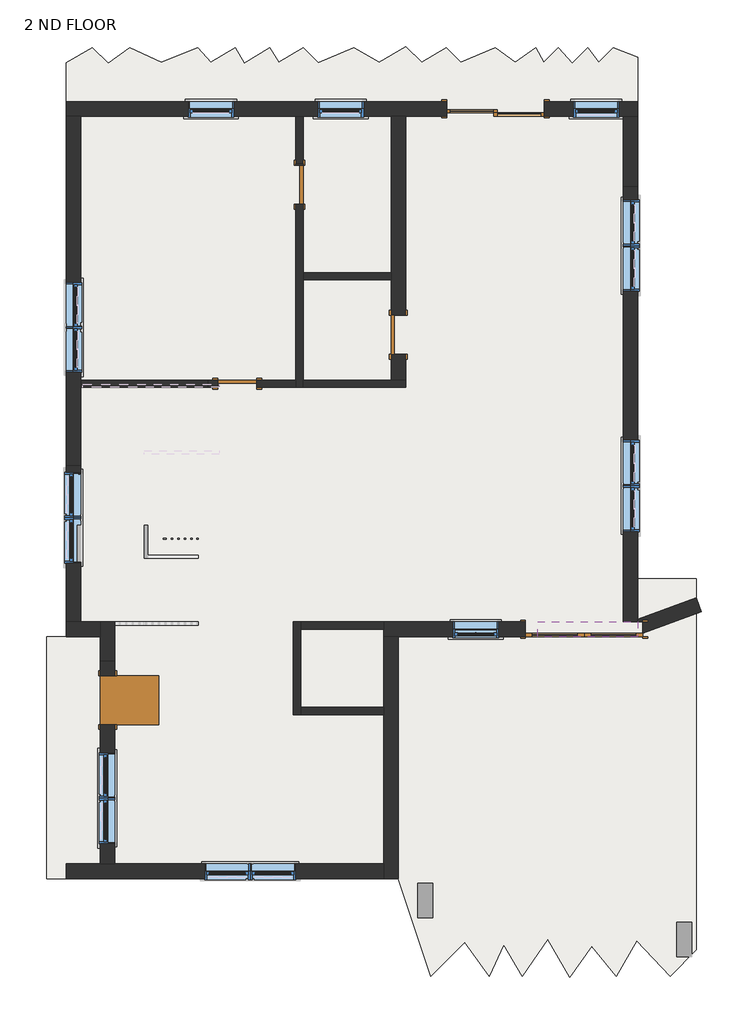
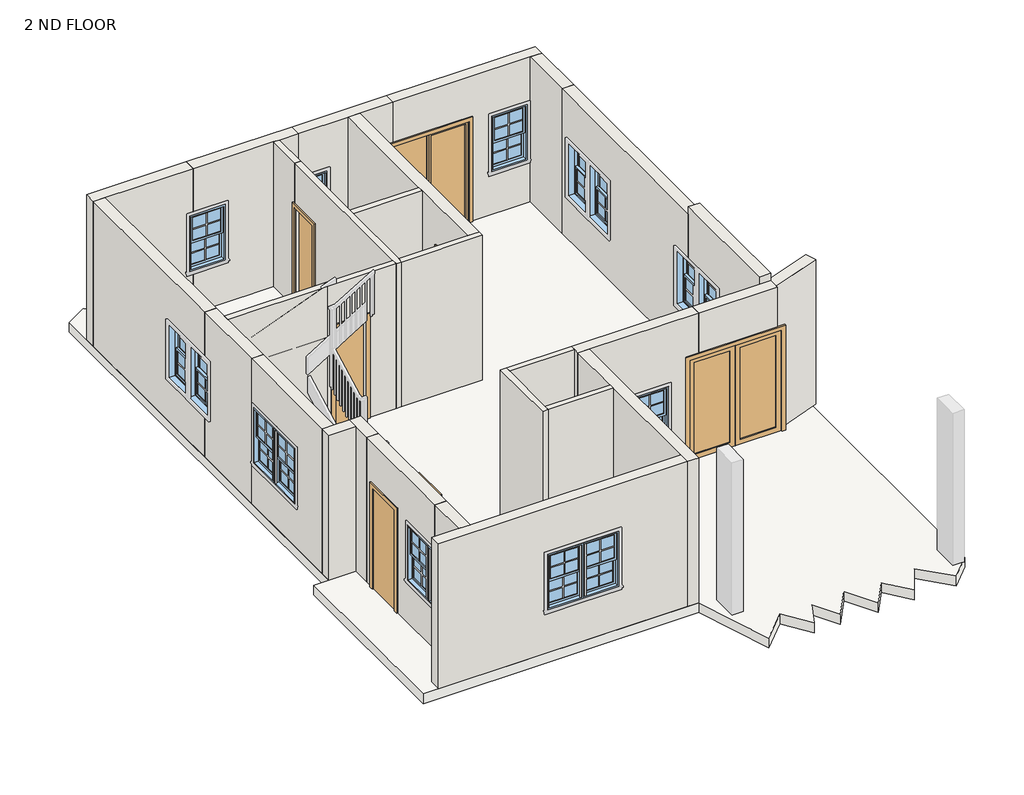
# One storey, part 1 of 3: 29 walls, 16 windows, 6 doors, 1 slab.
"""IFC4 building model written with IfcOpenShell, lengths in millimetres."""

from ifc_helpers import new_model, si_unit, frame, origin, place, context, project, spatial, polyline, outline, extrude, faceted_brep, transform, mapped, element, save
from components import door_5cbd26dd, door_238c678e, single_flush_2_x_7_f433b8c7, door_0bf9f8da, door_0d3b4037, window_fc4bf0c6

model = new_model("IFC4")

# Units and contexts
model_context = context("Model", 3, world=origin())
ifc_project = project(units=[si_unit("LENGTHUNIT", "METRE", prefix="MILLI")], contexts=[model_context])

# Site, building, storey
site = spatial("IfcSite", under=ifc_project)
building = spatial("IfcBuilding", under=site)
storey = spatial("IfcBuildingStorey", under=building, Name="2 ND FLOOR", Elevation=6400.8)

# Doors
placement = place(None, origin())
door_shape = door_5cbd26dd(model_context)
element("IfcDoor", 1, ObjectType="Door-Double-Glass : 72\" x 84\"", at=placement, inside=storey, context=model_context, shape_type="MappedRepresentation", body=[
    mapped(door_shape, transform((-14398.9750992, 4551.4036146, 6400.8), x_axis=(-1.0, 0.0, 0.0), y_axis=(0.0, -1.0, 0.0), z_axis=(0.0, 0.0, 1.0))),
])
door_2_shape = door_238c678e(model_context)
element("IfcDoor", 2, ObjectType="Door-Double-Sliding : 60\" x 84\"", at=placement, inside=storey, context=model_context, shape_type="MappedRepresentation", body=[
    mapped(door_2_shape, transform((-15781.8310804, 12791.3223147, 6400.8), x_axis=(-1.0, 0.0, 0.0), y_axis=(0.0, -1.0, 0.0), z_axis=(0.0, 0.0, 1.0))),
])
single_flush_2_x_7_shape = single_flush_2_x_7_f433b8c7(model_context)
element("IfcDoor", 3, ObjectType="Single-Flush : 2' x 7'", at=placement, inside=storey, context=model_context, shape_type="MappedRepresentation", body=[
    mapped(single_flush_2_x_7_shape, transform((-21828.4750314, 3444.1223646, 6400.8), x_axis=(0.0, 1.0, 0.0), y_axis=(-1.0, 0.0, 0.0), z_axis=(0.0, 0.0, 1.0))),
])
door_3_shape = door_0bf9f8da(model_context)
element("IfcDoor", 4, ObjectType="Single-Flush : 24\" x 84\"", at=placement, inside=storey, context=model_context, shape_type="MappedRepresentation", body=[
    mapped(door_3_shape, transform((-18837.6250314, 11478.1423646, 6400.8), x_axis=(0.0, 1.0, 0.0), y_axis=(-1.0, 0.0, 0.0), z_axis=(0.0, 0.0, 1.0))),
])
element("IfcDoor", 5, ObjectType="Single-Flush : 24\" x 84\"", at=placement, inside=storey, context=model_context, shape_type="MappedRepresentation", body=[
    mapped(door_3_shape, transform((-19809.1750314, 8378.0723646, 6400.8), x_axis=(-1.0, 0.0, 0.0), y_axis=(0.0, -1.0, 0.0), z_axis=(0.0, 0.0, 1.0))),
])
door_4_shape = door_0d3b4037(model_context)
element("IfcDoor", 6, ObjectType="Single-Flush : 24\" x 84\"", at=placement, inside=storey, context=model_context, shape_type="MappedRepresentation", body=[
    mapped(door_4_shape, transform((-17294.5750314, 9140.0723646, 6400.8), x_axis=(0.0, 1.0, 0.0), y_axis=(-1.0, 0.0, 0.0), z_axis=(0.0, 0.0, 1.0))),
])

# Slab
element("IfcSlab", 7, ObjectType="LW Concrete on Metal Deck", at=placement, inside=storey, context=model_context, shape_type="SweptSolid", body=[
    extrude(outline(polyline([(-22065.2814022, 13616.8223646), (-21820.2943548, 13371.8353173), (-21483.0986122, 13616.8223646), (-20992.8643301, 13388.2223646), (-20427.0594754, 13616.8223646), (-20220.0943548, 13388.2223646), (-19839.6400652, 13616.8223646), (-19695.738427, 13377.3298208), (-19297.1559002, 13616.8223646), (-19159.7991627, 13388.2223646), (-18779.344873, 13616.8223646), (-18543.6943548, 13381.1718464), (-17988.5365241, 13616.8223646), (-17592.5897095, 13388.2223646), (-17180.2750314, 13635.9660173), (-16932.5313787, 13388.2223646), (-16552.077089, 13616.8223646), (-16323.477089, 13388.2223646), (-15784.9292382, 13616.8223646), (-15470.2883312, 13388.2223646), (-15155.6474241, 13616.8223646), (-15028.932375, 13388.2223646), (-14800.332375, 13616.8223646), (-14581.2943548, 13373.5559982), (-14338.0279884, 13616.8223646), (-14171.9403665, 13388.2223646), (-13943.3403665, 13616.8223646), (-13560.7750314, 13469.9692914), (-13560.7750314, 5336.4223722), (-12646.3750314, 5336.4223722), (-12646.3750314, -450.2583119), (-13057.2943548, -861.1776354), (-13577.9943548, -311.251504), (-13895.4943548, -861.1776354), (-14276.4943548, -390.1805798), (-14619.3943548, -879.8925313), (-14962.2943548, -285.9723094), (-15365.0574601, -861.1776354), (-15648.0943548, -370.9433534), (-15876.6943548, -861.1776354), (-16257.6943548, -327.7776354), (-16791.0943548, -861.1776354), (-17294.5750314, 662.8223646), (-22780.9751188, 662.8223646), (-22780.9751188, 4434.7223646), (-22476.1752061, 4434.7223646), (-22476.1752061, 13379.5927163), (-22065.2814022, 13616.8223646)])), frame((0.0, 0.0, 6197.6), z_axis=(0.0, 0.0, 1.0), x_axis=(1.0, 0.0, 0.0)), (0.0, 0.0, 1.0), 203.2),
])

# Walls
element("IfcWall", 8, ObjectType="Generic - 4.5\"", at=placement, inside=storey, context=model_context, shape_type="SweptSolid", body=[
    extrude(outline(polyline([(-18894.7750314, 11808.3423646), (-18894.7750314, 12550.0223147), (-18780.4750314, 12550.0223147), (-18780.4750314, 11808.3423646), (-18894.7750314, 11808.3423646)])), frame((0.0, 0.0, 6400.8), z_axis=(0.0, 0.0, 1.0), x_axis=(1.0, 0.0, 0.0)), (0.0, 0.0, 1.0), 3048.0),
])
element("IfcWall", 9, ObjectType="Generic - 4.5\"", at=placement, inside=storey, context=model_context, shape_type="Brep", body=[
    faceted_brep([(-18894.7750314, 11808.3423646, 6400.8), (-18894.7750314, 11782.9423646, 6400.8), (-18894.7750314, 11782.9423646, 8534.4), (-18894.7750314, 11173.3423646, 8534.4), (-18894.7750314, 11173.3423646, 6400.8), (-18894.7750314, 8435.2223646, 6400.8), (-18894.7750314, 8320.9223646, 6400.8), (-18894.7750314, 8320.9223646, 9448.8), (-18894.7750314, 8435.2223646, 9448.8), (-18894.7750314, 11808.3423646, 9448.8), (-18780.4750314, 11782.9423646, 8534.4), (-18780.4750314, 11782.9423646, 6400.8), (-18780.4750314, 11808.3423646, 6400.8), (-18780.4750314, 11808.3423646, 9448.8), (-18780.4750314, 10111.6223646, 9448.8), (-18780.4750314, 9997.3223646, 9448.8), (-18780.4750314, 8435.2223646, 9448.8), (-18780.4750314, 8320.9223646, 9448.8), (-18780.4750314, 8320.9223646, 6400.8), (-18780.4750314, 8435.2223646, 6400.8), (-18780.4750314, 9997.3223646, 6400.8), (-18780.4750314, 10111.6223646, 6400.8), (-18780.4750314, 11173.3423646, 6400.8), (-18780.4750314, 11173.3423646, 8534.4)], [[[0, 1, 2, 3, 4, 5, 6, 7, 8, 9]], [[10, 11, 12, 13, 14, 15, 16, 17, 18, 19, 20, 21, 22, 23]], [[12, 11, 1, 0]], [[22, 21, 20, 19, 18, 6, 5, 4]], [[9, 8, 7, 17, 16, 15, 14, 13]], [[0, 9, 13, 12]], [[7, 6, 18, 17]], [[2, 1, 11, 10]], [[3, 2, 10, 23]], [[4, 3, 23, 22]]]),
])
element("IfcWall", 10, ObjectType="Generic - 4.5\"", at=placement, inside=storey, context=model_context, shape_type="Brep", body=[
    faceted_brep([(-18780.4750314, 8320.9223646, 6400.8), (-17180.2750314, 8320.9223646, 6400.8), (-17180.2750314, 8320.9223646, 9448.8), (-18780.4750314, 8320.9223646, 9448.8), (-18780.4750314, 8435.2223646, 6400.8), (-18780.4750314, 8435.2223646, 9448.8), (-17408.8750314, 8435.2223646, 9448.8), (-17180.2750314, 8435.2223646, 9448.8), (-17180.2750314, 8435.2223646, 6400.8), (-17408.8750314, 8435.2223646, 6400.8)], [[[0, 1, 2, 3]], [[4, 5, 6, 7, 8, 9]], [[1, 0, 4, 9, 8]], [[3, 2, 7, 6, 5]], [[0, 3, 5, 4]], [[2, 1, 8, 7]]]),
])
element("IfcWall", 11, ObjectType="Generic - 4.5\"", at=placement, inside=storey, context=model_context, shape_type="SweptSolid", body=[
    extrude(outline(polyline([(6400.8, -20266.3750314), (6400.8, -20113.9750314), (8534.4, -20113.9750314), (8534.4, -19504.3750314), (6400.8, -19504.3750314), (6400.8, -18894.7750314), (9448.8, -18894.7750314), (9448.8, -20266.3750314), (6400.8, -20266.3750314)])), frame((0.0, 8320.9223646, 0.0), z_axis=(0.0, 1.0, 0.0), x_axis=(0.0, 0.0, 1.0)), (0.0, 0.0, 1.0), 114.3),
])
element("IfcWall", 12, ObjectType="Generic - 4.5\"", at=placement, inside=storey, context=model_context, shape_type="SweptSolid", body=[
    extrude(outline(polyline([(-20266.3750314, 8320.9223646), (-22247.5752061, 8320.9223646), (-22247.5752061, 8435.2223646), (-20266.3750314, 8435.2223646), (-20266.3750314, 8320.9223646)])), frame((0.0, 0.0, 6400.8), z_axis=(0.0, 0.0, 1.0), x_axis=(1.0, 0.0, 0.0)), (0.0, 0.0, 1.0), 3048.0),
])
element("IfcWall", 13, ObjectType="Generic - 4.5\"", at=placement, inside=storey, context=model_context, shape_type="SweptSolid", body=[
    extrude(outline(polyline([(-17408.8750314, 9997.3223646), (-18780.4750314, 9997.3223646), (-18780.4750314, 10111.6223646), (-17408.8750314, 10111.6223646), (-17408.8750314, 9997.3223646)])), frame((0.0, 0.0, 6400.8), z_axis=(0.0, 0.0, 1.0), x_axis=(1.0, 0.0, 0.0)), (0.0, 0.0, 1.0), 3048.0),
])
element("IfcWall", 14, ObjectType="Generic - 4.5\"", at=placement, inside=storey, context=model_context, shape_type="Brep", body=[
    faceted_brep([(-18932.8750314, 4663.3223646, 6400.8), (-18932.8750314, 3215.5223646, 6400.8), (-18932.8750314, 3215.5223646, 9448.8), (-18932.8750314, 4663.3223646, 9448.8), (-18818.5750314, 4663.3223646, 6400.8), (-18818.5750314, 4663.3223646, 9448.8), (-18818.5750314, 4549.0223646, 9448.8), (-18818.5750314, 3329.8223646, 9448.8), (-18818.5750314, 3215.5223646, 9448.8), (-18818.5750314, 3215.5223646, 6400.8), (-18818.5750314, 3329.8223646, 6400.8), (-18818.5750314, 4549.0223646, 6400.8)], [[[0, 1, 2, 3]], [[4, 5, 6, 7, 8, 9, 10, 11]], [[1, 0, 4, 11, 10, 9]], [[3, 2, 8, 7, 6, 5]], [[2, 1, 9, 8]], [[0, 3, 5, 4]]]),
])
element("IfcWall", 15, ObjectType="Generic - 4.5\"", at=placement, inside=storey, context=model_context, shape_type="SweptSolid", body=[
    extrude(outline(polyline([(-17523.1750314, 3215.5223646), (-18818.5750314, 3215.5223646), (-18818.5750314, 3329.8223646), (-17523.1750314, 3329.8223646), (-17523.1750314, 3215.5223646)])), frame((0.0, 0.0, 6400.8), z_axis=(0.0, 0.0, 1.0), x_axis=(1.0, 0.0, 0.0)), (0.0, 0.0, 1.0), 3048.0),
])
element("IfcWall", 16, ObjectType="Generic - 4.5\"", at=placement, inside=storey, context=model_context, shape_type="SweptSolid", body=[
    extrude(outline(polyline([(-17523.1750314, 4549.0223646), (-18818.5750314, 4549.0223646), (-18818.5750314, 4663.3223646), (-17523.1750314, 4663.3223646), (-17523.1750314, 4549.0223646)])), frame((0.0, 0.0, 6400.8), z_axis=(0.0, 0.0, 1.0), x_axis=(1.0, 0.0, 0.0)), (0.0, 0.0, 1.0), 3048.0),
])
element("IfcWall", 17, ObjectType="Generic -9\"Brick 2", at=placement, inside=storey, context=model_context, shape_type="Brep", body=[
    faceted_brep([(-22476.1750314, 12550.0223646, 6400.8), (-22247.5750314, 12550.0223646, 6400.8), (-20494.9750314, 12550.0223646, 6400.8), (-20494.9750314, 12550.0223646, 7315.2), (-20571.1750314, 12550.0223646, 7315.2), (-20571.1750314, 12550.0223646, 8483.6), (-20494.9750314, 12550.0223646, 8483.6), (-20494.9750314, 12550.0223646, 9448.8), (-22247.5750314, 12550.0223646, 9448.8), (-22476.1750314, 12550.0223646, 9448.8), (-20494.9750314, 12778.6223646, 6400.8), (-22476.1750314, 12778.6223646, 6400.8), (-22476.1750314, 12778.6223646, 9448.8), (-20494.9750314, 12778.6223646, 9448.8), (-20494.9750314, 12778.6223646, 8483.6), (-20571.1750314, 12778.6223646, 8483.6), (-20571.1750314, 12778.6223646, 7315.2), (-20494.9750314, 12778.6223646, 7315.2)], [[[0, 1, 2, 3, 4, 5, 6, 7, 8, 9]], [[10, 11, 12, 13, 14, 15, 16, 17]], [[2, 1, 0, 11, 10]], [[2, 10, 17, 3]], [[13, 7, 6, 14]], [[9, 8, 7, 13, 12]], [[0, 9, 12, 11]], [[16, 4, 3, 17]], [[4, 16, 15, 5]], [[5, 15, 14, 6]]]),
])
element("IfcWall", 18, ObjectType="Generic -9\"Brick 2", at=placement, inside=storey, context=model_context, shape_type="Brep", body=[
    faceted_brep([(-20494.9750314, 12550.0223147, 6400.8), (-18894.7750314, 12550.0223147, 6400.8), (-18780.4750314, 12550.0223147, 6400.8), (-18397.0494379, 12550.0223147, 6400.8), (-18397.0494379, 12550.0223147, 7315.2), (-18549.4494379, 12550.0223147, 7315.2), (-18549.4494379, 12550.0223147, 8483.6), (-18397.0494379, 12550.0223147, 8483.6), (-18397.0494379, 12550.0223147, 9448.8), (-18780.4750314, 12550.0223147, 9448.8), (-18894.7750314, 12550.0223147, 9448.8), (-20494.9750314, 12550.0223147, 9448.8), (-20494.9750314, 12550.0223147, 8483.6), (-19859.9750314, 12550.0223147, 8483.6), (-19859.9750314, 12550.0223147, 7315.2), (-20494.9750314, 12550.0223147, 7315.2), (-18397.0494379, 12778.6223147, 6400.8), (-20494.9750314, 12778.6223147, 6400.8), (-20494.9750314, 12778.6223147, 7315.2), (-19859.9750314, 12778.6223147, 7315.2), (-19859.9750314, 12778.6223147, 8483.6), (-20494.9750314, 12778.6223147, 8483.6), (-20494.9750314, 12778.6223147, 9448.8), (-18397.0494379, 12778.6223147, 9448.8), (-18397.0494379, 12778.6223147, 8483.6), (-18549.4494379, 12778.6223147, 8483.6), (-18549.4494379, 12778.6223147, 7315.2), (-18397.0494379, 12778.6223147, 7315.2)], [[[0, 1, 2, 3, 4, 5, 6, 7, 8, 9, 10, 11, 12, 13, 14, 15]], [[16, 17, 18, 19, 20, 21, 22, 23, 24, 25, 26, 27]], [[3, 2, 1, 0, 17, 16]], [[3, 16, 27, 4]], [[23, 8, 7, 24]], [[11, 10, 9, 8, 23, 22]], [[11, 22, 21, 12]], [[17, 0, 15, 18]], [[13, 20, 19, 14]], [[14, 19, 18, 15]], [[20, 13, 12, 21]], [[26, 5, 4, 27]], [[5, 26, 25, 6]], [[6, 25, 24, 7]]]),
])
element("IfcWall", 19, ObjectType="Generic -9\"Brick 2", at=placement, inside=storey, context=model_context, shape_type="Brep", body=[
    faceted_brep([(-16518.4310804, 12550.0223147, 9448.8), (-17180.2750314, 12550.0223147, 9448.8), (-17408.8750314, 12550.0223147, 9448.8), (-18397.0494379, 12550.0223147, 9448.8), (-18397.0494379, 12550.0223147, 8483.6), (-17838.2494379, 12550.0223147, 8483.6), (-17838.2494379, 12550.0223147, 7315.2), (-18397.0494379, 12550.0223147, 7315.2), (-18397.0494379, 12550.0223147, 6400.8), (-17408.8750314, 12550.0223147, 6400.8), (-17180.2750314, 12550.0223147, 6400.8), (-16543.8310804, 12550.0223147, 6400.8), (-16543.8310804, 12550.0223147, 8534.4), (-16518.4310804, 12550.0223147, 8534.4), (-18397.0494379, 12778.6223147, 9448.8), (-16518.4310804, 12778.6223147, 9448.8), (-16518.4310804, 12778.6223147, 8534.4), (-16543.8310804, 12778.6223147, 8534.4), (-16543.8310804, 12778.6223147, 6400.8), (-18397.0494379, 12778.6223147, 6400.8), (-18397.0494379, 12778.6223147, 7315.2), (-17838.2494379, 12778.6223147, 7315.2), (-17838.2494379, 12778.6223147, 8483.6), (-18397.0494379, 12778.6223147, 8483.6)], [[[0, 1, 2, 3, 4, 5, 6, 7, 8, 9, 10, 11, 12, 13]], [[14, 15, 16, 17, 18, 19, 20, 21, 22, 23]], [[8, 19, 18, 11, 10, 9]], [[15, 0, 13, 16]], [[3, 2, 1, 0, 15, 14]], [[3, 14, 23, 4]], [[19, 8, 7, 20]], [[5, 22, 21, 6]], [[6, 21, 20, 7]], [[22, 5, 4, 23]], [[17, 12, 11, 18]], [[12, 17, 16, 13]]]),
])
element("IfcWall", 20, ObjectType="Generic -9\"Brick 2", at=placement, inside=storey, context=model_context, shape_type="Brep", body=[
    faceted_brep([(-13560.7750314, 12550.0223147, 9448.8), (-13789.3750314, 12550.0223147, 9448.8), (-16518.4310804, 12550.0223147, 9448.8), (-16518.4310804, 12550.0223147, 8534.4), (-15019.8310804, 12550.0223147, 8534.4), (-15019.8310804, 12550.0223147, 6400.8), (-13789.3750314, 12550.0223147, 6400.8), (-13560.7750314, 12550.0223147, 6400.8), (-13852.8750314, 12550.0223147, 8483.6), (-13852.8750314, 12550.0223147, 7315.2), (-14564.0750314, 12550.0223147, 7315.2), (-14564.0750314, 12550.0223147, 8483.6), (-16518.4310804, 12778.6223147, 9448.8), (-13560.7750314, 12778.6223147, 9448.8), (-13560.7750314, 12778.6223147, 6400.8), (-15019.8310804, 12778.6223147, 6400.8), (-15019.8310804, 12778.6223147, 8534.4), (-16518.4310804, 12778.6223147, 8534.4), (-13852.8750314, 12778.6223147, 7315.2), (-13852.8750314, 12778.6223147, 8483.6), (-14564.0750314, 12778.6223147, 8483.6), (-14564.0750314, 12778.6223147, 7315.2)], [[[0, 1, 2, 3, 4, 5, 6, 7], [8, 9, 10, 11]], [[12, 13, 14, 15, 16, 17], [18, 19, 20, 21]], [[14, 7, 6, 5, 15]], [[2, 1, 0, 13, 12]], [[2, 12, 17, 3]], [[0, 7, 14, 13]], [[4, 16, 15, 5]], [[16, 4, 3, 17]], [[8, 19, 18, 9]], [[9, 18, 21, 10]], [[10, 21, 20, 11]], [[19, 8, 11, 20]]]),
])
element("IfcWall", 21, ObjectType="Generic -9\"Brick 2", at=placement, inside=storey, context=model_context, shape_type="SweptSolid", body=[
    extrude(outline(polyline([(-13789.3750314, 11447.1098201), (-13789.3750314, 12550.0223147), (-13560.7750314, 12550.0223147), (-13560.7750314, 11447.1098201), (-13789.3750314, 11447.1098201)])), frame((0.0, 0.0, 6400.8), z_axis=(0.0, 0.0, 1.0), x_axis=(1.0, 0.0, 0.0)), (0.0, 0.0, 1.0), 3048.0),
])
element("IfcWall", 22, ObjectType="Generic -9\"Brick 2", at=placement, inside=storey, context=model_context, shape_type="SweptSolid", body=[
    extrude(outline(polyline([(11447.1098201, 6400.8), (7101.7223647, 6400.8), (7101.7223647, 7315.2), (7495.4223646, 7315.2), (7495.4223646, 8483.6), (7101.7223647, 8483.6), (7101.7223647, 9448.8), (11447.1098201, 9448.8), (11447.1098201, 6400.8)]), holes=[polyline([(9821.5098201, 7315.2), (11243.9098201, 7315.2), (11243.9098201, 8483.6), (9821.5098201, 8483.6), (9821.5098201, 7315.2)])]), frame((-13789.3750314, 0.0, 0.0), z_axis=(1.0, 0.0, 0.0), x_axis=(0.0, 1.0, 0.0)), (0.0, 0.0, 1.0), 228.6),
])
element("IfcWall", 23, ObjectType="Generic -9\"Brick 2", at=placement, inside=storey, context=model_context, shape_type="Brep", body=[
    faceted_brep([(-13789.3750314, 7101.7223647, 6400.8), (-13789.3750314, 4663.3223646, 6400.8), (-13789.3750314, 4663.3223646, 9601.2), (-13789.3750314, 7101.7223647, 9601.2), (-13789.3750314, 7101.7223647, 9448.8), (-13789.3750314, 7101.7223647, 8483.6), (-13789.3750314, 6073.0223646, 8483.6), (-13789.3750314, 6073.0223646, 7315.2), (-13789.3750314, 7101.7223647, 7315.2), (-13560.7750314, 4663.3223646, 6400.8), (-13560.7750314, 4704.9241624, 6400.8), (-13560.7750314, 7101.7223647, 6400.8), (-13560.7750314, 7101.7223647, 7315.2), (-13560.7750314, 6073.0223646, 7315.2), (-13560.7750314, 6073.0223646, 8483.6), (-13560.7750314, 7101.7223647, 8483.6), (-13560.7750314, 7101.7223647, 9448.8), (-13560.7750314, 7101.7223647, 9601.2), (-13560.7750314, 4663.3223646, 9601.2), (-13560.7750314, 4663.3223646, 9448.8), (-13560.7750314, 4663.3223646, 8534.4)], [[[0, 1, 2, 3, 4, 5, 6, 7, 8]], [[9, 10, 11, 12, 13, 14, 15, 16, 17, 18, 19, 20]], [[1, 0, 11, 10, 9]], [[3, 2, 18, 17]], [[3, 17, 16, 15, 5, 4]], [[11, 0, 8, 12]], [[2, 1, 9, 20, 19, 18]], [[7, 13, 12, 8]], [[5, 15, 14, 6]], [[13, 7, 6, 14]]]),
])
element("IfcWall", 24, ObjectType="Generic -9\"Brick 2", at=placement, inside=storey, context=model_context, shape_type="Brep", body=[
    faceted_brep([(-13560.7750314, 4434.7223646, 9448.8), (-15122.8751671, 4434.7223646, 9448.8), (-15122.8751671, 4434.7223646, 8534.4), (-13560.7750314, 4434.7223646, 8534.4), (-15122.8751671, 4663.3223646, 9448.8), (-13560.7750314, 4663.3223646, 9448.8), (-13560.7750314, 4663.3223646, 8534.4), (-15122.8751671, 4663.3223646, 8534.4), (-13560.7750314, 4461.6531236, 9448.8), (-13560.7750314, 4461.6531236, 8534.4)], [[[0, 1, 2, 3]], [[4, 5, 6, 7]], [[1, 0, 8, 5, 4]], [[1, 4, 7, 2]], [[5, 8, 0, 3, 9, 6]], [[3, 2, 7, 6, 9]]]),
])
element("IfcWall", 25, ObjectType="Generic -9\"Brick 2", at=placement, inside=storey, context=model_context, shape_type="Brep", body=[
    faceted_brep([(-17523.1750314, 4663.3223722, 9448.8), (-15122.8751671, 4663.3223722, 9448.8), (-15122.8751671, 4663.3223722, 8534.4), (-15313.3750992, 4663.3223722, 8534.4), (-15313.3750992, 4663.3223722, 6400.8), (-17523.1750314, 4663.3223722, 6400.8), (-15732.4750314, 4663.3223722, 6961.9134602), (-15732.4750314, 4663.3223722, 8130.3134602), (-16443.6750314, 4663.3223722, 8130.3134602), (-16443.6750314, 4663.3223722, 6961.9134602), (-15122.8751671, 4434.7223722, 9448.8), (-17294.5750314, 4434.7223722, 9448.8), (-17523.1750314, 4434.7223722, 9448.8), (-17523.1750314, 4434.7223722, 6400.8), (-17294.5750314, 4434.7223722, 6400.8), (-15313.3750992, 4434.7223722, 6400.8), (-15313.3750992, 4434.7223722, 8534.4), (-15122.8751671, 4434.7223722, 8534.4), (-15732.4750314, 4434.7223722, 8130.3134602), (-15732.4750314, 4434.7223722, 6961.9134602), (-16443.6750314, 4434.7223722, 6961.9134602), (-16443.6750314, 4434.7223722, 8130.3134602), (-17523.1750314, 4549.0223646, 6400.8), (-17523.1750314, 4549.0223646, 9448.8)], [[[0, 1, 2, 3, 4, 5], [6, 7, 8, 9]], [[10, 11, 12, 13, 14, 15, 16, 17], [18, 19, 20, 21]], [[13, 22, 5, 4, 15, 14]], [[1, 0, 23, 12, 11, 10]], [[1, 10, 17, 2]], [[0, 5, 22, 13, 12, 23]], [[3, 16, 15, 4]], [[16, 3, 2, 17]], [[18, 7, 6, 19]], [[19, 6, 9, 20]], [[20, 9, 8, 21]], [[7, 18, 21, 8]]]),
])
element("IfcWall", 26, ObjectType="Generic -9\"Brick 2", at=placement, inside=storey, context=model_context, shape_type="Brep", body=[
    faceted_brep([(-17523.1750314, 4434.7223722, 6400.8), (-17523.1750314, 3329.8223646, 6400.8), (-17523.1750314, 3215.5223646, 6400.8), (-17523.1750314, 891.4223646, 6400.8), (-17523.1750314, 662.8223646, 6400.8), (-17523.1750314, 662.8223646, 9448.8), (-17523.1750314, 891.4223646, 9448.8), (-17523.1750314, 3215.5223646, 9448.8), (-17523.1750314, 3329.8223646, 9448.8), (-17523.1750314, 4434.7223722, 9448.8), (-17294.5750314, 4434.7223722, 6400.8), (-17294.5750314, 4434.7223722, 9448.8), (-17294.5750314, 662.8223646, 9448.8), (-17294.5750314, 662.8223646, 6400.8)], [[[0, 1, 2, 3, 4, 5, 6, 7, 8, 9]], [[10, 11, 12, 13]], [[4, 3, 2, 1, 0, 10, 13]], [[9, 8, 7, 6, 5, 12, 11]], [[0, 9, 11, 10]], [[5, 4, 13, 12]]]),
])
element("IfcWall", 27, ObjectType="Generic -9\"Brick 2", at=placement, inside=storey, context=model_context, shape_type="Brep", body=[
    faceted_brep([(-17523.1750314, 891.4223646, 6400.8), (-21714.1750314, 891.4223646, 6400.8), (-21942.7750314, 891.4223646, 6400.8), (-22476.1750314, 891.4223646, 6400.8), (-22476.1750314, 891.4223646, 9448.8), (-21942.7750314, 891.4223646, 9448.8), (-21714.1750314, 891.4223646, 9448.8), (-17523.1750314, 891.4223646, 9448.8), (-18894.6931686, 891.4223646, 8483.6), (-20317.0931686, 891.4223646, 8483.6), (-20317.0931686, 891.4223646, 7315.2), (-18894.6931686, 891.4223646, 7315.2), (-22476.1750314, 662.8223646, 6400.8), (-17523.1750314, 662.8223646, 6400.8), (-17523.1750314, 662.8223646, 9448.8), (-22476.1750314, 662.8223646, 9448.8), (-20317.0931686, 662.8223646, 8483.6), (-18894.6931686, 662.8223646, 8483.6), (-18894.6931686, 662.8223646, 7315.2), (-20317.0931686, 662.8223646, 7315.2)], [[[0, 1, 2, 3, 4, 5, 6, 7], [8, 9, 10, 11]], [[12, 13, 14, 15], [16, 17, 18, 19]], [[3, 2, 1, 0, 13, 12]], [[4, 3, 12, 15]], [[7, 6, 5, 4, 15, 14]], [[0, 7, 14, 13]], [[8, 17, 16, 9]], [[19, 10, 9, 16]], [[17, 8, 11, 18]], [[18, 11, 10, 19]]]),
])
element("IfcWall", 28, ObjectType="Generic -9\"Brick 2", at=placement, inside=storey, context=model_context, shape_type="SweptSolid", body=[
    extrude(outline(polyline([(1710.5723646, 6400.8), (891.4223646, 6400.8), (891.4223646, 9448.8), (1710.5723646, 9448.8), (1710.5723646, 8483.6), (1202.5723646, 8483.6), (1202.5723646, 7315.2), (1710.5723646, 7315.2), (1710.5723646, 6400.8)])), frame((-21942.7750314, 0.0, 0.0), z_axis=(1.0, 0.0, 0.0), x_axis=(0.0, 1.0, 0.0)), (0.0, 0.0, 1.0), 228.6),
])
element("IfcWall", 29, ObjectType="Generic -9\"Brick 2", at=placement, inside=storey, context=model_context, shape_type="SweptSolid", body=[
    extrude(outline(polyline([(1710.5723646, 9448.8), (4053.7223646, 9448.8), (4053.7223646, 6400.8), (3825.1223646, 6400.8), (3825.1223646, 8534.4), (3063.1223646, 8534.4), (3063.1223646, 6400.8), (1710.5723646, 6400.8), (1710.5723646, 7315.2), (2624.9723646, 7315.2), (2624.9723646, 8483.6), (1710.5723646, 8483.6), (1710.5723646, 9448.8)])), frame((-21942.7750314, 0.0, 0.0), z_axis=(1.0, 0.0, 0.0), x_axis=(0.0, 1.0, 0.0)), (0.0, 0.0, 1.0), 228.6),
])
element("IfcWall", 30, ObjectType="Generic -9\"Brick 2", at=placement, inside=storey, context=model_context, shape_type="Brep", body=[
    faceted_brep([(-21714.1750314, 4053.7223646, 6400.8), (-21714.1750314, 4663.3223646, 6400.8), (-21714.1750314, 4663.3223646, 9448.8), (-21714.1750314, 4053.7223646, 9448.8), (-21942.7750314, 4053.7223646, 6400.8), (-21942.7750314, 4053.7223646, 9448.8), (-21942.7750314, 4434.7223646, 9448.8), (-21942.7750314, 4663.3223646, 9448.8), (-21942.7750314, 4663.3223646, 6400.8), (-21942.7750314, 4434.7223646, 6400.8)], [[[0, 1, 2, 3]], [[4, 5, 6, 7, 8, 9]], [[1, 0, 4, 9, 8]], [[3, 2, 7, 6, 5]], [[0, 3, 5, 4]], [[2, 1, 8, 7]]]),
])
element("IfcWall", 31, ObjectType="Generic -9\"Brick 2", at=placement, inside=storey, context=model_context, shape_type="SweptSolid", body=[
    extrude(outline(polyline([(12550.0223646, 6400.8), (8710.539033, 6400.8), (8710.539033, 7315.2), (9955.139033, 7315.2), (9955.139033, 8483.6), (8710.539033, 8483.6), (8710.539033, 9448.8), (12550.0223646, 9448.8), (12550.0223646, 6400.8)])), frame((-22476.1750314, 0.0, 0.0), z_axis=(1.0, 0.0, 0.0), x_axis=(0.0, 1.0, 0.0)), (0.0, 0.0, 1.0), 228.6),
])
element("IfcWall", 32, ObjectType="Generic -9\"Brick 2", at=placement, inside=storey, context=model_context, shape_type="Brep", body=[
    faceted_brep([(-22476.1752061, 8710.539033, 6400.8), (-22476.1752061, 7101.7223643, 6400.8), (-22476.1752061, 7101.7223643, 9448.8), (-22476.1752061, 8710.539033, 9448.8), (-22476.1752061, 8710.539033, 8483.6), (-22476.1752061, 8558.139033, 8483.6), (-22476.1752061, 8558.139033, 7315.2), (-22476.1752061, 8710.539033, 7315.2), (-22247.5752061, 7101.7223643, 6400.8), (-22247.5752061, 8320.9223646, 6400.8), (-22247.5752061, 8435.2223646, 6400.8), (-22247.5752061, 8710.539033, 6400.8), (-22247.5752061, 8710.539033, 7315.2), (-22247.5752061, 8558.139033, 7315.2), (-22247.5752061, 8558.139033, 8483.6), (-22247.5752061, 8710.539033, 8483.6), (-22247.5752061, 8710.539033, 9448.8), (-22247.5752061, 8435.2223646, 9448.8), (-22247.5752061, 8320.9223646, 9448.8), (-22247.5752061, 7101.7223643, 9448.8)], [[[0, 1, 2, 3, 4, 5, 6, 7]], [[8, 9, 10, 11, 12, 13, 14, 15, 16, 17, 18, 19]], [[1, 0, 11, 10, 9, 8]], [[2, 1, 8, 19]], [[3, 2, 19, 18, 17, 16]], [[3, 16, 15, 4]], [[11, 0, 7, 12]], [[6, 13, 12, 7]], [[13, 6, 5, 14]], [[14, 5, 4, 15]]]),
])
element("IfcWall", 33, ObjectType="Generic -9\"Brick 2", at=placement, inside=storey, context=model_context, shape_type="SweptSolid", body=[
    extrude(outline(polyline([(7101.7223643, 6400.8), (4663.3223646, 6400.8), (4663.3223646, 9448.8), (7101.7223643, 9448.8), (7101.7223643, 6400.8)]), holes=[polyline([(5577.7223643, 7315.2), (7000.1223643, 7315.2), (7000.1223643, 8483.6), (5577.7223643, 8483.6), (5577.7223643, 7315.2)])]), frame((-22476.1752061, 0.0, 0.0), z_axis=(1.0, 0.0, 0.0), x_axis=(0.0, 1.0, 0.0)), (0.0, 0.0, 1.0), 228.6),
])
element("IfcWall", 34, ObjectType="Generic -9\"Brick 2", at=placement, inside=storey, context=model_context, shape_type="Brep", body=[
    faceted_brep([(-22476.1752061, 4434.7223646, 6400.8), (-21942.7750314, 4434.7223646, 6400.8), (-21942.7750314, 4434.7223646, 9448.8), (-22476.1752061, 4434.7223646, 9448.8), (-22476.1752061, 4663.3223646, 6400.8), (-22476.1752061, 4663.3223646, 9448.8), (-22247.5752061, 4663.3223646, 9448.8), (-21942.7750314, 4663.3223646, 9448.8), (-21942.7750314, 4663.3223646, 6400.8), (-22247.5752061, 4663.3223646, 6400.8)], [[[0, 1, 2, 3]], [[4, 5, 6, 7, 8, 9]], [[1, 0, 4, 9, 8]], [[3, 2, 7, 6, 5]], [[0, 3, 5, 4]], [[2, 1, 8, 7]]]),
])
element("IfcWall", 35, ObjectType="Generic -9\"Brick 2", at=placement, inside=storey, context=model_context, shape_type="Brep", body=[
    faceted_brep([(-17408.8750314, 12550.0223147, 6400.8), (-17408.8750314, 10111.6223646, 6400.8), (-17408.8750314, 9997.3223646, 6400.8), (-17408.8750314, 9444.8723646, 6400.8), (-17408.8750314, 9444.8723646, 8534.4), (-17408.8750314, 8835.2723646, 8534.4), (-17408.8750314, 8835.2723646, 6400.8), (-17408.8750314, 8435.2223646, 6400.8), (-17408.8750314, 8435.2223646, 9448.8), (-17408.8750314, 9997.3223646, 9448.8), (-17408.8750314, 10111.6223646, 9448.8), (-17408.8750314, 12550.0223147, 9448.8), (-17180.2750314, 9444.8723646, 8534.4), (-17180.2750314, 9444.8723646, 6400.8), (-17180.2750314, 12550.0223147, 6400.8), (-17180.2750314, 12550.0223147, 9448.8), (-17180.2750314, 8435.2223646, 9448.8), (-17180.2750314, 8435.2223646, 6400.8), (-17180.2750314, 8835.2723646, 6400.8), (-17180.2750314, 8835.2723646, 8534.4)], [[[0, 1, 2, 3, 4, 5, 6, 7, 8, 9, 10, 11]], [[12, 13, 14, 15, 16, 17, 18, 19]], [[18, 17, 7, 6]], [[14, 13, 3, 2, 1, 0]], [[11, 10, 9, 8, 16, 15]], [[0, 11, 15, 14]], [[8, 7, 17, 16]], [[4, 3, 13, 12]], [[5, 4, 12, 19]], [[6, 5, 19, 18]]]),
])
element("IfcWall", 36, ObjectType="Generic -9\"Brick 2", at=placement, inside=storey, context=model_context, shape_type="Brep", body=[
    faceted_brep([(-12570.5569462, 4822.063032, 6400.8), (-12570.5569462, 4822.063032, 9448.8), (-13560.7750314, 4461.6531236, 9448.8), (-13560.7750314, 4461.6531236, 8534.4), (-13484.5750992, 4489.3876307, 8534.4), (-13484.5750992, 4489.3876307, 6400.8), (-12648.7427509, 5036.8767651, 6400.8), (-13560.7750314, 4704.9241624, 6400.8), (-13560.7750314, 4704.9241624, 9448.8), (-12648.7427509, 5036.8767651, 9448.8), (-13484.5750992, 4663.3223646, 6400.8), (-13560.7750314, 4663.3223646, 6400.8), (-13560.7750314, 4663.3223646, 9448.8), (-13560.7750314, 4663.3223646, 8534.4), (-13484.5750992, 4663.3223646, 8534.4)], [[[0, 1, 2, 3, 4, 5]], [[6, 7, 8, 9]], [[7, 6, 0, 5, 10, 11]], [[1, 0, 6, 9]], [[2, 1, 9, 8, 12]], [[2, 12, 8, 7, 11, 13, 3]], [[14, 4, 3, 13]], [[14, 10, 5, 4]], [[10, 14, 13, 11]]]),
])

# Windows
window_shape = window_fc4bf0c6(model_context)
element("IfcWindow", 37, ObjectType="Window-Double-Hung : 28\" x 46\"", at=placement, inside=storey, context=model_context, shape_type="MappedRepresentation", body=[
    mapped(window_shape, transform((-20215.5750314, 12664.3223147, 6400.8), x_axis=(-1.0, 0.0, 0.0), y_axis=(0.0, -1.0, 0.0), z_axis=(0.0, 0.0, 1.0))),
])
element("IfcWindow", 38, ObjectType="Window-Double-Hung : 28\" x 46\"", at=placement, inside=storey, context=model_context, shape_type="MappedRepresentation", body=[
    mapped(window_shape, transform((-14208.4750314, 12664.3223147, 6400.8), x_axis=(-1.0, 0.0, 0.0), y_axis=(0.0, -1.0, 0.0), z_axis=(0.0, 0.0, 1.0))),
])
element("IfcWindow", 39, ObjectType="Window-Double-Hung : 28\" x 46\"", at=placement, inside=storey, context=model_context, shape_type="MappedRepresentation", body=[
    mapped(window_shape, transform((-13675.0750314, 10888.3098201, 6400.8), x_axis=(0.0, -1.0, 0.0), y_axis=(1.0, 0.0, 0.0), z_axis=(0.0, 0.0, 1.0))),
])
element("IfcWindow", 40, ObjectType="Window-Double-Hung : 28\" x 46\"", at=placement, inside=storey, context=model_context, shape_type="MappedRepresentation", body=[
    mapped(window_shape, transform((-13675.0750314, 10177.1098201, 6400.8), x_axis=(0.0, -1.0, 0.0), y_axis=(1.0, 0.0, 0.0), z_axis=(0.0, 0.0, 1.0))),
])
element("IfcWindow", 41, ObjectType="Window-Double-Hung : 28\" x 46\"", at=placement, inside=storey, context=model_context, shape_type="MappedRepresentation", body=[
    mapped(window_shape, transform((-13675.0750314, 7139.8223646, 6400.8), x_axis=(0.0, -1.0, 0.0), y_axis=(1.0, 0.0, 0.0), z_axis=(0.0, 0.0, 1.0))),
])
element("IfcWindow", 42, ObjectType="Window-Double-Hung : 28\" x 46\"", at=placement, inside=storey, context=model_context, shape_type="MappedRepresentation", body=[
    mapped(window_shape, transform((-13675.0750314, 6428.6223646, 6400.8), x_axis=(0.0, -1.0, 0.0), y_axis=(1.0, 0.0, 0.0), z_axis=(0.0, 0.0, 1.0))),
])
element("IfcWindow", 43, ObjectType="Window-Double-Hung : 28\" x 46\"", at=placement, inside=storey, context=model_context, shape_type="MappedRepresentation", body=[
    mapped(window_shape, transform((-19961.4931686, 777.1223646, 6400.8), x_axis=(-1.0, 0.0, 0.0), y_axis=(0.0, -1.0, 0.0), z_axis=(0.0, 0.0, 1.0))),
])
element("IfcWindow", 44, ObjectType="Window-Double-Hung : 28\" x 46\"", at=placement, inside=storey, context=model_context, shape_type="MappedRepresentation", body=[
    mapped(window_shape, transform((-19250.2931686, 777.1223646, 6400.8), x_axis=(-1.0, 0.0, 0.0), y_axis=(0.0, -1.0, 0.0), z_axis=(0.0, 0.0, 1.0))),
])
element("IfcWindow", 45, ObjectType="Window-Double-Hung : 28\" x 46\"", at=placement, inside=storey, context=model_context, shape_type="MappedRepresentation", body=[
    mapped(window_shape, transform((-21828.4750314, 2269.3723646, 6400.8), x_axis=(0.0, 1.0, 0.0), y_axis=(-1.0, 0.0, 0.0), z_axis=(0.0, 0.0, 1.0))),
])
element("IfcWindow", 46, ObjectType="Window-Double-Hung : 28\" x 46\"", at=placement, inside=storey, context=model_context, shape_type="MappedRepresentation", body=[
    mapped(window_shape, transform((-21828.4750314, 1558.1723646, 6400.8), x_axis=(0.0, 1.0, 0.0), y_axis=(-1.0, 0.0, 0.0), z_axis=(0.0, 0.0, 1.0))),
])
element("IfcWindow", 47, ObjectType="Window-Double-Hung : 28\" x 46\"", at=placement, inside=storey, context=model_context, shape_type="MappedRepresentation", body=[
    mapped(window_shape, transform((-22361.8752061, 6644.5223643, 6400.8), x_axis=(0.0, 1.0, 0.0), y_axis=(-1.0, 0.0, 0.0), z_axis=(0.0, 0.0, 1.0))),
])
element("IfcWindow", 48, ObjectType="Window-Double-Hung : 28\" x 46\"", at=placement, inside=storey, context=model_context, shape_type="MappedRepresentation", body=[
    mapped(window_shape, transform((-22361.8752061, 5933.3223643, 6400.8), x_axis=(0.0, 1.0, 0.0), y_axis=(-1.0, 0.0, 0.0), z_axis=(0.0, 0.0, 1.0))),
])
element("IfcWindow", 49, ObjectType="Window-Double-Hung : 28\" x 46\"", at=placement, inside=storey, context=model_context, shape_type="MappedRepresentation", body=[
    mapped(window_shape, transform((-22361.8750314, 9599.539033, 6400.8), x_axis=(0.0, -1.0, 0.0), y_axis=(1.0, 0.0, 0.0), z_axis=(0.0, 0.0, 1.0))),
])
element("IfcWindow", 50, ObjectType="Window-Double-Hung : 28\" x 46\"", at=placement, inside=storey, context=model_context, shape_type="MappedRepresentation", body=[
    mapped(window_shape, transform((-22361.8750314, 8913.739033, 6400.8), x_axis=(0.0, -1.0, 0.0), y_axis=(1.0, 0.0, 0.0), z_axis=(0.0, 0.0, 1.0))),
])
element("IfcWindow", 51, ObjectType="Window-Double-Hung : 28\" x 46\"", at=placement, inside=storey, context=model_context, shape_type="MappedRepresentation", body=[
    mapped(window_shape, transform((-18193.8494379, 12664.3223147, 6400.8), x_axis=(-1.0, 0.0, 0.0), y_axis=(0.0, -1.0, 0.0), z_axis=(0.0, 0.0, 1.0))),
])
element("IfcWindow", 52, ObjectType="Window-Double-Hung : 28\" x 46\"", at=placement, inside=storey, context=model_context, shape_type="MappedRepresentation", body=[
    mapped(window_shape, transform((-16088.0750314, 4549.0223722, 6047.5134602), x_axis=(-1.0, 0.0, 0.0), y_axis=(0.0, -1.0, 0.0), z_axis=(0.0, 0.0, 1.0))),
])

save(model, "model.ifc")

# Revit data of these elements
# Type "Door-Double-Glass : 72\" x 84\""
#   Type Mark = "13"
#   Construction Type Id = "opn-d45"
#   Assembly Code = "C1020"
#   Analytic Construction = "Wood frame, double glass door "
#   W = 3' - 0"
#   Thickness = 0' - 2"
#   Thermal Resistance (R) = 1.8150 (h·ft²·°F)/BTU
#   Swing Angle [instance default] = 90.00°
#   Heat Transfer Coefficient (U) = 0.5510 BTU/(h·ft²·°F)
#   Height = 7' - 0"
#   Bottom Rail = 0' - 4"
#   Top Rail = 0' - 4"
#   Stiles = 0' - 4"
#   Trim Projection = 0' - 1"
#   Trim Width = 0' - 3"
#   Width = 6' - 0"
#   Define Thermal Properties by = 1
#   Glazing = Glass
#   Panel Material = Wood - Birch - Solid Stained Light Low Gloss
#   Trim Material = Paint - Sienna
#   Visual Light Transmittance = 0
#   Solar Heat Gain Coefficient = 0
#   Function = (empty or 0)
#   Wall Closure = (empty or 0)
# Type "Door-Double-Sliding : 60\" x 84\""
#   Type Mark = "9"
#   Construction Type Id = "opn-d45"
#   Assembly Code = "C1020"
#   Analytic Construction = "Wood frame, double glass door "
#   Thickness = 0' - 2"
#   Thermal Resistance (R) = 1.8150 (h·ft²·°F)/BTU
#   Heat Transfer Coefficient (U) = 0.5510 BTU/(h·ft²·°F)
#   Height = 7' - 0"
#   Rail Width = 0' - 2"
#   Stiles = 0' - 2"
#   Trim Projection Ext = 0' - 1"
#   Trim Projection Int = 0' - 1"
#   Trim Width = 0' - 3"
#   Width = 5' - 0"
#   Define Thermal Properties by = 1
#   Glazing = Glass
#   Panel Material = Wood - Birch - Solid Stained Light Low Gloss
#   Trim Material = Paint - Sienna
#   Visual Light Transmittance = 0
#   Solar Heat Gain Coefficient = 0
#   Function = (empty or 0)
#   Wall Closure = (empty or 0)
# Type "Single-Flush : 2' x 7'"
#   Type Mark = "10"
#   Construction Type Id = "MDOOR"
#   Assembly Code = "C1020"
#   Analytic Construction = "Metal"
#   Thickness = 3' - 0"
#   Heat Transfer Coefficient (U) = 0.651978 BTU/(h·ft²·°F)
#   Height = 7' - 0"
#   Trim Projection Ext = 0' - 1"
#   Trim Projection Int = 0' - 1"
#   Trim Width = 0' - 3"
#   Width = 2' - 6"
#   Define Thermal Properties by = 1
#   Door Material = Door - Panel
#   Frame Material = Door - Frame
#   Visual Light Transmittance = 0
#   Solar Heat Gain Coefficient = 0
#   Function = (empty or 0)
#   Wall Closure = (empty or 0)
# Type "Single-Flush : 24\" x 84\""
#   Type Mark = "1"
#   Construction Type Id = "MDOOR"
#   Assembly Code = "C1020"
#   Analytic Construction = "Metal"
#   Thickness = 0' - 2"
#   Heat Transfer Coefficient (U) = 0.651978 BTU/(h·ft²·°F)
#   Height = 7' - 0"
#   Trim Projection Ext = 0' - 1"
#   Trim Projection Int = 0' - 1"
#   Trim Width = 0' - 3"
#   Width = 2' - 0"
#   Define Thermal Properties by = 1
#   Define Thermal Properties by = 1
#   Door Material = Door - Panel
#   Frame Material = Door - Frame
#   Visual Light Transmittance = 0
#   Solar Heat Gain Coefficient = 0
#   Function = (empty or 0)
#   Wall Closure = (empty or 0)
# Type "LW Concrete on Metal Deck"
#   Assembly Code = "B1010"
#   Function = 0
#   Layers, outside or top first: 0' - 6" "Concrete, Lightweight" (function 1); 0' - 2" "Metal Deck" (function 1)
# Type "Generic - 4.5\""
#   Assembly Code = "B2010"
#   Layers, outside or top first: 0' - 4 1/2" no material (function 1)
# Type "Generic -9\"Brick 2"
#   Assembly Code = "B2010"
#   Layers, outside or top first: 0' - 9" "Brick, Common" (function 1)
# Type "Window-Double-Hung : 28\" x 46\""
#   Type Mark = "12"
#   Fire Rating = "0.5h"
#   Construction Type Id = "DG-DR"
#   Assembly Code = "B2020100"
#   Analytic Construction = "Double glazing - domestic"
#   Wall Thickness [instance default] = 0' - 6"
#   Window Inset [instance default] = 0' - 0"
#   Visual Light Transmittance = 0.81
#   Thermal Resistance (R) = 1.8146 (h·ft²·°F)/BTU
#   Solar Heat Gain Coefficient = 0.76
#   Muntin Width = 1' - 10"
#   Muntin Height = 1' - 7 1/8"
#   Interior Wall Closure [instance default] = 0' - 1 1/2"
#   Rough Width = 2' - 4 1/2"
#   Rough Height = 3' - 10 1/2"
#   Frame Extension [instance default] = 0' - 1 1/4"
#   Exterior Wall Closure [instance default] = 0' - 0 1/2"
#   Extension Jamb [instance default] = 0' - 1 1/2"
#   Heat Transfer Coefficient (U) = 0.5511 BTU/(h·ft²·°F)
#   Height = 3' - 10"
#   Width = 2' - 4"
#   Define Thermal Properties by = 1
#   Top Muntin Visibility = yes
#   Indicator Visibility [instance default] = yes
#   Extension Jamb Visibility [instance default] = yes
#   Interior Trim Visibility [instance default] = yes
#   Exterior Trim Visibility [instance default] = yes
#   Define Thermal Properties by = 1
#   Bottom Muntin Visibility = yes
#   Muntin Pattern = Muntin Pattern_2x2 : Muntin Pattern_2x2
#   Interior Trim Material = Wood - Stained
#   Interior Trim = Trim-Window-Interior-Flat : Picture Frame
#   Exterior Trim Material = Clad - White
#   Exterior Trim = Trim-Window-Exterior-Flat : with Sill
#   Glass Panel Material = Glass
#   Exterior Frame Material = Clad - White
#   Interior Frame Material = Wood - Stained
#   Wall Closure = (empty or 0)
# Element 1 (IfcDoor, "Door-Double-Glass : 72\" x 84\"")
#   Swing Angle = 90.00°
#   Phase Created = New Construction
#   Materials on its faces: "Wood - Birch - Solid Stained Light Low Gloss", "Paint - Sienna", "Glass"
# Element 2 (IfcDoor, "Door-Double-Sliding : 60\" x 84\"")
#   Phase Created = New Construction
#   Materials on its faces: "Paint - Sienna", "Wood - Birch - Solid Stained Light Low Gloss", "Glass"
# Element 3 (IfcDoor, "Single-Flush : 2' x 7'")
#   Phase Created = New Construction
#   Materials on its faces: "Door - Frame", "Door - Panel"
# Elements 4, 5, 6 (IfcDoor, "Single-Flush : 24\" x 84\"")
#   Phase Created = New Construction
#   Materials on its faces: "Door - Frame", "Door - Panel"
# Element 7 (IfcSlab, "LW Concrete on Metal Deck")
#   built-in parameter 1001955 = -1.5708 (stored number, unit not read)
#   Height Offset From Level = 0' - 0"
#   Phase Created = New Construction
#   Materials on its faces: "Metal Deck", "Concrete, Lightweight"
# Elements 8, 9, 11, 12, 13, 14, 15, 16 (IfcWall, "Generic - 4.5\"")
#   Top Offset = 10' - 0"
#   Base Offset = 0' - 0"
#   wall height = 10' - 0"
#   Phase Created = New Construction
#   Base Constraint = 2 ND FLOOR
#   Top Constraint = 2 ND FLOOR
#   Materials on its faces: "Default Wall"
# Element 10 (IfcWall, "Generic - 4.5\"")
#   Top Offset = 10' - 0"
#   Base Offset = 0' - 0"
#   wall height = 10' - 0"
#   Phase Created = New Construction
#   Base Constraint = 2 ND FLOOR
#   Top Constraint = 2 ND FLOOR
#   Materials on its faces: "Default Wall", "Brick, Common"
# Elements 17, 18, 19, 20, 21, 22, 24, 25, 26, 27, 28, 29, 30, 31, 32, 33, 34, 35, 36 (IfcWall, "Generic -9\"Brick 2")
#   Top Offset = 10' - 0"
#   Base Offset = 0' - 0"
#   wall height = 10' - 0"
#   Phase Created = New Construction
#   Base Constraint = 2 ND FLOOR
#   Top Constraint = 2 ND FLOOR
#   Materials on its faces: "Brick, Common"
# Element 23 (IfcWall, "Generic -9\"Brick 2")
#   Top Offset = 10' - 6"
#   Base Offset = 0' - 0"
#   wall height = 10' - 6"
#   Phase Created = New Construction
#   Base Constraint = 2 ND FLOOR
#   Top Constraint = 2 ND FLOOR
#   Materials on its faces: "Brick, Common"
# Element 37 (IfcWindow, "Window-Double-Hung : 28\" x 46\"")
#   Mark = "32"
#   Window Inset = 0' - 0"
#   Interior Wall Closure = 0' - 1 1/2"
#   Frame Extension = 0' - 1 1/4"
#   Exterior Wall Closure = 0' - 0 1/2"
#   Interior Trim Visibility = yes
#   Indicator Visibility = yes
#   Exterior Trim Visibility = yes
#   Phase Created = New Construction
#   Materials on its faces: "Wood - Stained", "Glass", "Clad - White"
# Element 38 (IfcWindow, "Window-Double-Hung : 28\" x 46\"")
#   Mark = "33"
#   Window Inset = 0' - 0"
#   Interior Wall Closure = 0' - 1 1/2"
#   Frame Extension = 0' - 1 1/4"
#   Exterior Wall Closure = 0' - 0 1/2"
#   Interior Trim Visibility = yes
#   Indicator Visibility = yes
#   Exterior Trim Visibility = yes
#   Phase Created = New Construction
#   Materials on its faces: "Wood - Stained", "Glass", "Clad - White"
# Element 39 (IfcWindow, "Window-Double-Hung : 28\" x 46\"")
#   Mark = "34"
#   Window Inset = 0' - 0"
#   Interior Wall Closure = 0' - 1 1/2"
#   Frame Extension = 0' - 1 1/4"
#   Exterior Wall Closure = 0' - 0 1/2"
#   Interior Trim Visibility = yes
#   Indicator Visibility = yes
#   Exterior Trim Visibility = yes
#   Phase Created = New Construction
#   Materials on its faces: "Wood - Stained", "Glass", "Clad - White"
# Element 40 (IfcWindow, "Window-Double-Hung : 28\" x 46\"")
#   Mark = "35"
#   Window Inset = 0' - 0"
#   Interior Wall Closure = 0' - 1 1/2"
#   Frame Extension = 0' - 1 1/4"
#   Exterior Wall Closure = 0' - 0 1/2"
#   Interior Trim Visibility = yes
#   Indicator Visibility = yes
#   Exterior Trim Visibility = yes
#   Phase Created = New Construction
#   Materials on its faces: "Wood - Stained", "Glass", "Clad - White"
# Element 41 (IfcWindow, "Window-Double-Hung : 28\" x 46\"")
#   Mark = "36"
#   Window Inset = 0' - 0"
#   Interior Wall Closure = 0' - 1 1/2"
#   Frame Extension = 0' - 1 1/4"
#   Exterior Wall Closure = 0' - 0 1/2"
#   Interior Trim Visibility = yes
#   Indicator Visibility = yes
#   Exterior Trim Visibility = yes
#   Phase Created = New Construction
#   Materials on its faces: "Wood - Stained", "Glass", "Clad - White"
# Element 42 (IfcWindow, "Window-Double-Hung : 28\" x 46\"")
#   Mark = "37"
#   Window Inset = 0' - 0"
#   Interior Wall Closure = 0' - 1 1/2"
#   Frame Extension = 0' - 1 1/4"
#   Exterior Wall Closure = 0' - 0 1/2"
#   Interior Trim Visibility = yes
#   Indicator Visibility = yes
#   Exterior Trim Visibility = yes
#   Phase Created = New Construction
#   Materials on its faces: "Wood - Stained", "Glass", "Clad - White"
# Element 43 (IfcWindow, "Window-Double-Hung : 28\" x 46\"")
#   Mark = "38"
#   Window Inset = 0' - 0"
#   Interior Wall Closure = 0' - 1 1/2"
#   Frame Extension = 0' - 1 1/4"
#   Exterior Wall Closure = 0' - 0 1/2"
#   Interior Trim Visibility = yes
#   Indicator Visibility = yes
#   Exterior Trim Visibility = yes
#   Phase Created = New Construction
#   Materials on its faces: "Wood - Stained", "Glass", "Clad - White"
# Element 44 (IfcWindow, "Window-Double-Hung : 28\" x 46\"")
#   Mark = "39"
#   Window Inset = 0' - 0"
#   Interior Wall Closure = 0' - 1 1/2"
#   Frame Extension = 0' - 1 1/4"
#   Exterior Wall Closure = 0' - 0 1/2"
#   Interior Trim Visibility = yes
#   Indicator Visibility = yes
#   Exterior Trim Visibility = yes
#   Phase Created = New Construction
#   Materials on its faces: "Wood - Stained", "Glass", "Clad - White"
# Element 45 (IfcWindow, "Window-Double-Hung : 28\" x 46\"")
#   Mark = "40"
#   Window Inset = 0' - 0"
#   Interior Wall Closure = 0' - 1 1/2"
#   Frame Extension = 0' - 1 1/4"
#   Exterior Wall Closure = 0' - 0 1/2"
#   Interior Trim Visibility = yes
#   Indicator Visibility = yes
#   Exterior Trim Visibility = yes
#   Phase Created = New Construction
#   Materials on its faces: "Wood - Stained", "Glass", "Clad - White"
# Element 46 (IfcWindow, "Window-Double-Hung : 28\" x 46\"")
#   Mark = "41"
#   Window Inset = 0' - 0"
#   Interior Wall Closure = 0' - 1 1/2"
#   Frame Extension = 0' - 1 1/4"
#   Exterior Wall Closure = 0' - 0 1/2"
#   Interior Trim Visibility = yes
#   Indicator Visibility = yes
#   Exterior Trim Visibility = yes
#   Phase Created = New Construction
#   Materials on its faces: "Wood - Stained", "Glass", "Clad - White"
# Element 47 (IfcWindow, "Window-Double-Hung : 28\" x 46\"")
#   Mark = "42"
#   Window Inset = 0' - 0"
#   Interior Wall Closure = 0' - 1 1/2"
#   Frame Extension = 0' - 1 1/4"
#   Exterior Wall Closure = 0' - 0 1/2"
#   Interior Trim Visibility = yes
#   Indicator Visibility = yes
#   Exterior Trim Visibility = yes
#   Phase Created = New Construction
#   Materials on its faces: "Wood - Stained", "Glass", "Clad - White"
# Element 48 (IfcWindow, "Window-Double-Hung : 28\" x 46\"")
#   Mark = "43"
#   Window Inset = 0' - 0"
#   Interior Wall Closure = 0' - 1 1/2"
#   Frame Extension = 0' - 1 1/4"
#   Exterior Wall Closure = 0' - 0 1/2"
#   Interior Trim Visibility = yes
#   Indicator Visibility = yes
#   Exterior Trim Visibility = yes
#   Phase Created = New Construction
#   Materials on its faces: "Wood - Stained", "Glass", "Clad - White"
# Element 49 (IfcWindow, "Window-Double-Hung : 28\" x 46\"")
#   Mark = "44"
#   Window Inset = 0' - 0"
#   Interior Wall Closure = 0' - 1 1/2"
#   Frame Extension = 0' - 1 1/4"
#   Exterior Wall Closure = 0' - 0 1/2"
#   Interior Trim Visibility = yes
#   Indicator Visibility = yes
#   Exterior Trim Visibility = yes
#   Phase Created = New Construction
#   Materials on its faces: "Wood - Stained", "Glass", "Clad - White"
# Element 50 (IfcWindow, "Window-Double-Hung : 28\" x 46\"")
#   Mark = "45"
#   Window Inset = 0' - 0"
#   Interior Wall Closure = 0' - 1 1/2"
#   Frame Extension = 0' - 1 1/4"
#   Exterior Wall Closure = 0' - 0 1/2"
#   Interior Trim Visibility = yes
#   Indicator Visibility = yes
#   Exterior Trim Visibility = yes
#   Phase Created = New Construction
#   Materials on its faces: "Wood - Stained", "Glass", "Clad - White"
# Element 51 (IfcWindow, "Window-Double-Hung : 28\" x 46\"")
#   Mark = "46"
#   Window Inset = 0' - 0"
#   Interior Wall Closure = 0' - 1 1/2"
#   Frame Extension = 0' - 1 1/4"
#   Exterior Wall Closure = 0' - 0 1/2"
#   Interior Trim Visibility = yes
#   Indicator Visibility = yes
#   Exterior Trim Visibility = yes
#   Phase Created = New Construction
#   Materials on its faces: "Wood - Stained", "Glass", "Clad - White"
# Element 52 (IfcWindow, "Window-Double-Hung : 28\" x 46\"")
#   Mark = "49"
#   Window Inset = 0' - 0"
#   Interior Wall Closure = 0' - 1 1/2"
#   Frame Extension = 0' - 1 1/4"
#   Exterior Wall Closure = 0' - 0 1/2"
#   Interior Trim Visibility = yes
#   Indicator Visibility = yes
#   Exterior Trim Visibility = yes
#   Phase Created = New Construction
#   Materials on its faces: "Wood - Stained", "Glass", "Clad - White"
# Materials
#   "Glass": class "Glass", colour RGB 0 128 192, transparency 0.75, Description = "Soda Lime Glass", Cost = 0
#   "Wood - Birch - Solid Stained Light Low Gloss": class "Wood", colour RGB 210 159 95, transparency 0, Cost = 0
#   "Paint - Sienna": colour RGB 118 70 51, transparency 0, Cost = 0
#   "Door - Panel": class "Wood", colour RGB 210 159 95, transparency 0, Cost = 0
#   "Door - Frame": colour RGB 118 70 51, transparency 0, Cost = 0
#   "Concrete, Lightweight": class "Concrete", colour RGB 142 141 140, transparency 0, Description = "Lightweight concrete", Cost = 0
#   "Metal Deck": class "Metal", colour RGB 199 199 199, transparency 0, Description = "Steel, mill finish", Cost = 0
#   "Brick, Common": class "Masonry", colour RGB 170 98 104, transparency 0, Description = "Common brick", Cost = 0
#   "Wood - Stained": class "Wood", colour RGB 224 178 126, transparency 0, Cost = 0
#   "Clad - White": class "Wood", colour RGB 242 242 238, transparency 0, Cost = 0
#   "Default Wall": colour RGB 128 128 128, transparency 0, Cost = 0
